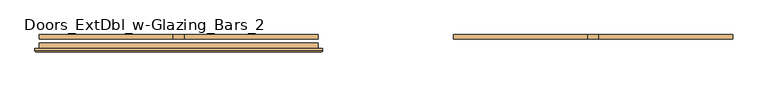
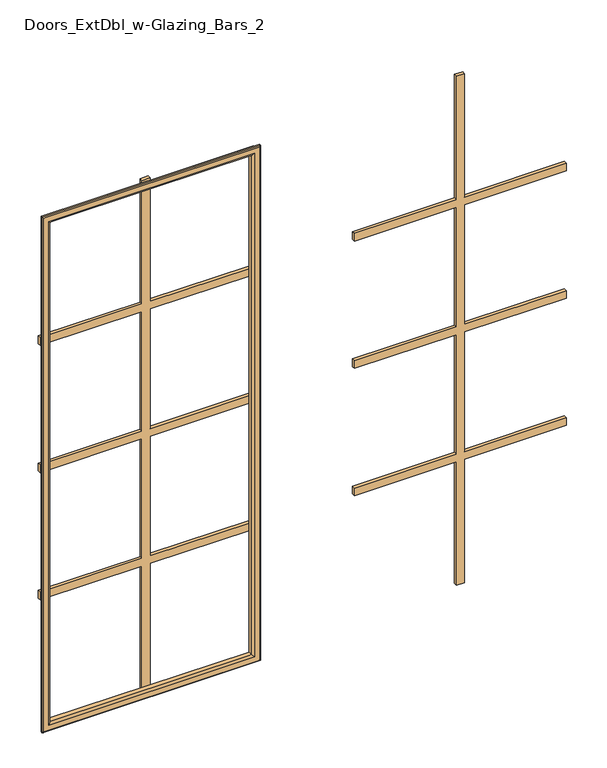
"""IFC4 building model written with IfcOpenShell, lengths in millimetres: door geometry, Doors_ExtDbl_w-Glazing_Bars_2."""

from ifc_helpers import new_model, si_unit, frame, origin, place, context, project, spatial, polyline, ellipse_curve, outline, extrude, source, transform, mapped, element, save
from ifc_brep_helpers import plane_surface, cylinder_surface, advanced_brep


def doors_extdbl_w_glazing_bars_2_fbc7e696(model_context):
    return source(origin(), model_context, "Body", "SolidModel", [
        advanced_brep(
        [(-656.5, -3.7, 1966.5), (-656.5, 0.3, 1966.5), (-656.5, 0.3, 625.5), (-656.5, -3.7, 625.5), (-654.5, -5.7, 1964.5), (-654.5, -5.7, 627.5), (-636.5, -0.7, 1946.5), (-641.5, -5.7, 1951.5), (-641.5, -5.7, 640.5), (-636.5, -0.7, 645.5), (-636.5, 10.3, 1946.5), (-636.5, 10.3, 645.5), (-648.5, 0.3, 1958.5), (-648.5, 10.3, 1958.5), (-648.5, 10.3, 633.5), (-648.5, 0.3, 633.5), (-118.5, 0.3, 625.5), (-118.5, -3.7, 625.5), (-120.5, -5.7, 627.5), (-133.5, -5.7, 640.5), (-138.5, -0.7, 645.5), (-138.5, 10.3, 645.5), (-126.5, 10.3, 633.5), (-126.5, 0.3, 633.5), (-118.5, 0.3, 1966.5), (-118.5, -3.7, 1966.5), (-120.5, -5.7, 1964.5), (-133.5, -5.7, 1951.5), (-138.5, -0.7, 1946.5), (-138.5, 10.3, 1946.5), (-126.5, 10.3, 1958.5), (-126.5, 0.3, 1958.5)],
        [
            (0, 1),
            (1, 2),
            (2, 3),
            (3, 0),
            (4, 0, ellipse_curve(frame((-654.5, -3.7, 1964.5), z_axis=(-0.7071067811865428, 0.0, -0.7071067811865522), x_axis=(-0.7071067811865523, 0.0, 0.7071067811865428)), 2.8284271, 2.0)),
            (3, 5, ellipse_curve(frame((-654.5, -3.7, 627.5), z_axis=(-0.7071067811865521, 0.0, 0.7071067811865428), x_axis=(0.7071067811865427, 0.0, 0.7071067811865523)), 2.8284271, 2.0)),
            (5, 4),
            (6, 7, ellipse_curve(frame((-641.5, -0.7, 1951.5), z_axis=(-0.7071067811865428, 0.0, -0.7071067811865522), x_axis=(-0.7071067811865523, 0.0, 0.7071067811865428)), 7.0710678, 5.0)),
            (7, 8),
            (8, 9, ellipse_curve(frame((-641.5, -0.7, 640.5), z_axis=(-0.7071067811865521, 0.0, 0.7071067811865428), x_axis=(0.7071067811865427, 0.0, 0.7071067811865523)), 7.0710678, 5.0)),
            (9, 6),
            (10, 6),
            (9, 11),
            (11, 10),
            (12, 13),
            (13, 14),
            (14, 15),
            (15, 12),
            (2, 16),
            (16, 17),
            (17, 3),
            (17, 18, ellipse_curve(frame((-120.5, -3.7, 627.5), z_axis=(-0.7071067811865428, 0.0, -0.7071067811865521), x_axis=(-0.7071067811865522, 0.0, 0.7071067811865427)), 2.8284271, 2.0)),
            (18, 5),
            (8, 19),
            (19, 20, ellipse_curve(frame((-133.5, -0.7, 640.5), z_axis=(-0.7071067811865428, 0.0, -0.7071067811865521), x_axis=(-0.7071067811865522, 0.0, 0.7071067811865427)), 7.0710678, 5.0)),
            (20, 9),
            (20, 21),
            (21, 11),
            (14, 22),
            (22, 23),
            (23, 15),
            (16, 24),
            (24, 25),
            (25, 17),
            (25, 26, ellipse_curve(frame((-120.5, -3.7, 1964.5), z_axis=(0.7071067811865523, 0.0, -0.7071067811865427), x_axis=(-0.7071067811865428, 0.0, -0.7071067811865523)), 2.8284271, 2.0)),
            (26, 18),
            (19, 27),
            (27, 28, ellipse_curve(frame((-133.5, -0.7, 1951.5), z_axis=(0.7071067811865523, 0.0, -0.7071067811865427), x_axis=(-0.7071067811865428, 0.0, -0.7071067811865523)), 7.0710678, 5.0)),
            (28, 20),
            (28, 29),
            (29, 21),
            (22, 30),
            (30, 31),
            (31, 23),
            (24, 1),
            (0, 25),
            (4, 26),
            (7, 27),
            (6, 28),
            (10, 29),
            (13, 30),
            (12, 31),
        ],
        [
            plane_surface(frame((-656.5, 0.3, 1966.5), z_axis=(-1.0, 0.0, 0.0), x_axis=(0.0, 0.0, -1.0))),
            cylinder_surface(frame((-654.5, -3.7, 1958.5), z_axis=(0.0, 0.0, 1.0), x_axis=(-1.0, 0.0, 0.0)), 2.0),
            cylinder_surface(frame((-641.5, -0.7, 1958.5), z_axis=(0.0, 0.0, 1.0), x_axis=(-1.0, 0.0, 0.0)), 5.0),
            plane_surface(frame((-636.5, -0.7, 1946.5), z_axis=(1.0, 0.0, 0.0), x_axis=(0.0, 0.0, -1.0))),
            plane_surface(frame((-648.5, 10.3, 1958.5), z_axis=(-1.0, 0.0, 0.0), x_axis=(0.0, 0.0, -1.0))),
            plane_surface(frame((-656.5, 0.3, 625.5), z_axis=(0.0, 0.0, -1.0), x_axis=(1.0, 0.0, 0.0))),
            cylinder_surface(frame((-648.5, -3.7, 627.5), z_axis=(-1.0, 0.0, 0.0), x_axis=(0.0, 0.0, -1.0)), 2.0),
            cylinder_surface(frame((-648.5, -0.7, 640.5), z_axis=(-1.0, 0.0, 0.0), x_axis=(0.0, 0.0, -1.0)), 5.0),
            plane_surface(frame((-636.5, -0.7, 645.5), z_axis=(0.0, 0.0, 1.0), x_axis=(1.0, 0.0, 0.0))),
            plane_surface(frame((-648.5, 10.3, 633.5), z_axis=(0.0, 0.0, -1.0), x_axis=(1.0, 0.0, 0.0))),
            plane_surface(frame((-118.5, 0.3, 625.5), z_axis=(1.0, 0.0, 0.0), x_axis=(0.0, 0.0, 1.0))),
            cylinder_surface(frame((-120.5, -3.7, 633.5), z_axis=(0.0, 0.0, -1.0), x_axis=(1.0, 0.0, 0.0)), 2.0),
            cylinder_surface(frame((-133.5, -0.7, 633.5), z_axis=(0.0, 0.0, -1.0), x_axis=(1.0, 0.0, 0.0)), 5.0),
            plane_surface(frame((-138.5, -0.7, 645.5), z_axis=(-1.0, 0.0, 0.0), x_axis=(0.0, 0.0, 1.0))),
            plane_surface(frame((-126.5, 10.3, 633.5), z_axis=(1.0, 0.0, 0.0), x_axis=(0.0, 0.0, 1.0))),
            plane_surface(frame((-118.5, 0.3, 1966.5), z_axis=(0.0, 0.0, 1.0), x_axis=(-1.0, 0.0, 0.0))),
            cylinder_surface(frame((-126.5, -3.7, 1964.5), z_axis=(1.0, 0.0, 0.0), x_axis=(0.0, 0.0, 1.0)), 2.0),
            plane_surface(frame((-120.5, -5.7, 1964.5), z_axis=(0.0, -1.0, 0.0), x_axis=(-1.0, 0.0, 0.0))),
            cylinder_surface(frame((-126.5, -0.7, 1951.5), z_axis=(1.0, 0.0, 0.0), x_axis=(0.0, 0.0, 1.0)), 5.0),
            plane_surface(frame((-138.5, -0.7, 1946.5), z_axis=(0.0, 0.0, -1.0), x_axis=(-1.0, 0.0, 0.0))),
            plane_surface(frame((-138.5, 10.3, 1946.5), z_axis=(0.0, 1.0, 0.0), x_axis=(-1.0, 0.0, 0.0))),
            plane_surface(frame((-126.5, 10.3, 1958.5), z_axis=(0.0, 0.0, 1.0), x_axis=(-1.0, 0.0, 0.0))),
            plane_surface(frame((-126.5, 0.3, 1958.5), z_axis=(0.0, 1.0, 0.0), x_axis=(-1.0, 0.0, 0.0))),
        ],
        [
            (0, [[1, 2, 3, 4]]),
            (1, [[5, -4, 6, 7]]),
            (2, [[8, 9, 10, 11]]),
            (3, [[12, -11, 13, 14]]),
            (4, [[15, 16, 17, 18]]),
            (5, [[-3, 19, 20, 21]]),
            (6, [[-6, -21, 22, 23]]),
            (7, [[-10, 24, 25, 26]]),
            (8, [[-13, -26, 27, 28]]),
            (9, [[-17, 29, 30, 31]]),
            (10, [[-20, 32, 33, 34]]),
            (11, [[-22, -34, 35, 36]]),
            (12, [[-25, 37, 38, 39]]),
            (13, [[-27, -39, 40, 41]]),
            (14, [[-30, 42, 43, 44]]),
            (15, [[-33, 45, -1, 46]]),
            (16, [[-35, -46, -5, 47]]),
            (17, [[-23, -36, -47, -7], [48, -37, -24, -9]]),
            (18, [[-38, -48, -8, 49]]),
            (19, [[-40, -49, -12, 50]]),
            (20, [[51, -42, -29, -16], [-28, -41, -50, -14]]),
            (21, [[-43, -51, -15, 52]]),
            (22, [[-45, -32, -19, -2], [-31, -44, -52, -18]]),
        ],
    ),
        extrude(outline(polyline([(1637.25, -377.5), (1958.5, -377.5), (1958.5, -397.5), (1637.25, -397.5), (1637.25, -648.5), (1617.25, -648.5), (1617.25, -397.5), (1306.0, -397.5), (1306.0, -648.5), (1286.0, -648.5), (1286.0, -397.5), (974.75, -397.5), (974.75, -648.5), (954.75, -648.5), (954.75, -397.5), (633.5, -397.5), (633.5, -377.5), (954.75, -377.5), (954.75, -126.5), (974.75, -126.5), (974.75, -377.5), (1286.0, -377.5), (1286.0, -126.5), (1306.0, -126.5), (1306.0, -377.5), (1617.25, -377.5), (1617.25, -126.5), (1637.25, -126.5), (1637.25, -377.5)])), frame((0.0, 18.3, 0.0), z_axis=(0.0, 1.0, 0.0), x_axis=(0.0, 0.0, 1.0)), (0.0, 0.0, 1.0), 8.0),
        extrude(outline(polyline([(1637.25, 397.5), (1958.5, 397.5), (1958.5, 377.5), (1637.25, 377.5), (1637.25, 126.5), (1617.25, 126.5), (1617.25, 377.5), (1306.0, 377.5), (1306.0, 126.5), (1286.0, 126.5), (1286.0, 377.5), (974.75, 377.5), (974.75, 126.5), (954.75, 126.5), (954.75, 377.5), (633.5, 377.5), (633.5, 397.5), (954.75, 397.5), (954.75, 648.5), (974.75, 648.5), (974.75, 397.5), (1286.0, 397.5), (1286.0, 648.5), (1306.0, 648.5), (1306.0, 397.5), (1617.25, 397.5), (1617.25, 648.5), (1637.25, 648.5), (1637.25, 397.5)])), frame((0.0, 18.3, 0.0), z_axis=(0.0, 1.0, 0.0), x_axis=(0.0, 0.0, 1.0)), (0.0, 0.0, 1.0), 8.0),
    ])


if __name__ == "__main__":
    model = new_model("IFC4")
    model_context = context("Model", 3, world=origin())
    ifc_project = project(units=[si_unit("LENGTHUNIT", "METRE", prefix="MILLI")], contexts=[model_context])
    site = spatial("IfcSite", under=ifc_project)
    building = spatial("IfcBuilding", under=site)
    placement = place(None, origin())
    doors_extdbl_w_glazing_bars_2_shape = doors_extdbl_w_glazing_bars_2_fbc7e696(model_context)
    element("IfcDoor", 1, ObjectType="Doors_ExtDbl_w-Glazing_Bars_2", at=placement, inside=building, context=model_context, shape_type="MappedRepresentation", body=[
        mapped(doors_extdbl_w_glazing_bars_2_shape, transform((0.0, 0.0, 0.0), x_axis=(1.0, 0.0, 0.0), y_axis=(0.0, 1.0, 0.0), z_axis=(0.0, 0.0, 1.0))),
    ])
    save(model, "model.ifc")

# Revit data of these elements
# Type "Doors_ExtDbl_w-Glazing_Bars_2"
#   Type Mark = "53"
#   Type Comments = "External Double"
#   Operation = "DoubleDoorSingleSwing"
#   Construction Type Id = "GSP4R"
#   Keynote = "L20"
#   Analytic Construction = "1/8 in Pilkington single glazing"
#   Wrap Layers (Int) from Ext = 0.1775 m
#   Wrap Layers (Ext) from Ext = 0.1025 m
#   Visual Light Transmittance = 0.9
#   Top of Intermediate Rail = 0.575 m
#   Thickness = 0.044 m
#   Stile Shutting = 0.125 m
#   Stile - Top Rail = 0.1 m
#   Stile - Lock Rail = 0.1 m
#   Stile - Hanging = 0.1 m
#   Stile - Bottom Rail = 0.175 m
#   Solar Heat Gain Coefficient = 0.78
#   Rough Width = 1.6 m
#   Rough Height = 2.11 m
#   O/A Frame Width = 0.064 m
#   Heat Transfer Coefficient (U) = 3.6886 W/(m²·K)
#   Handle Z Distance = 1.05 m
#   Glazing Thickness = 0.024 m
#   Glazing Bar Thickness = 0.02 m
#   FrameWidth = 0.042 m
#   FrameOffset - External = 0.025 m
#   FrameDepth = 0.089 m
#   Door Panel Width = 0.747 m
#   Door Panel Thickness = 0.044 m
#   Door Panel Height = 2.0 m
#   Cill Thickness = 0.0545 m
#   Cill Projection = 0.03 m
#   Handle X Distance = 0.075 m
#   Height = 2.11 m
#   Structural Tolerance = 0.0065 m
#   Tolerance = 0.003 m
#   Undercut = 0.004 m
#   Width = 1.6 m
#   Cill Extension = 0.025 m
#   Cavity Closer Width = 0.05 m
#   Cavity Closer Offset from Ext = 0.1025 m
#   Cavity Closer Depth = 0.085 m
#   Vis - Ironmongery = yes
#   Vis - Glazing Bars = yes
#   Vis - Cavity Closers = yes
#   Define Thermal Properties by = 1
#   Function = 1
#   Material Glazing Bars = Door - Panel
#   Material Glass = Door - Glazing
#   Material Door = Door - Panel
#   Material Frame = Door - Frame/Mullion
#   Material Ironmongery = Door - Handle
#   Wall Closure = (empty or 0)
#   Assembly Code = ""
# Element 1 (IfcDoor, "Doors_ExtDbl_w-Glazing_Bars_2")
#   Materials on its faces: "Door - Panel", "Door - Handle", "Door - Frame/Mullion", "Door - Glazing"
# Materials
#   "Door - Panel": class "Wood", colour RGB 210 159 95, transparency 0, Keynote = "L20", Cost = 0
#   "Door - Glazing": colour RGB 0 0 255, transparency 0.75
#   "Door - Frame/Mullion": class "Wood", colour RGB 212 179 113, transparency 0, Keynote = "L20", Cost = 0
#   "Door - Handle": colour RGB 0 0 0, transparency 0, Keynote = "P21", Cost = 0
